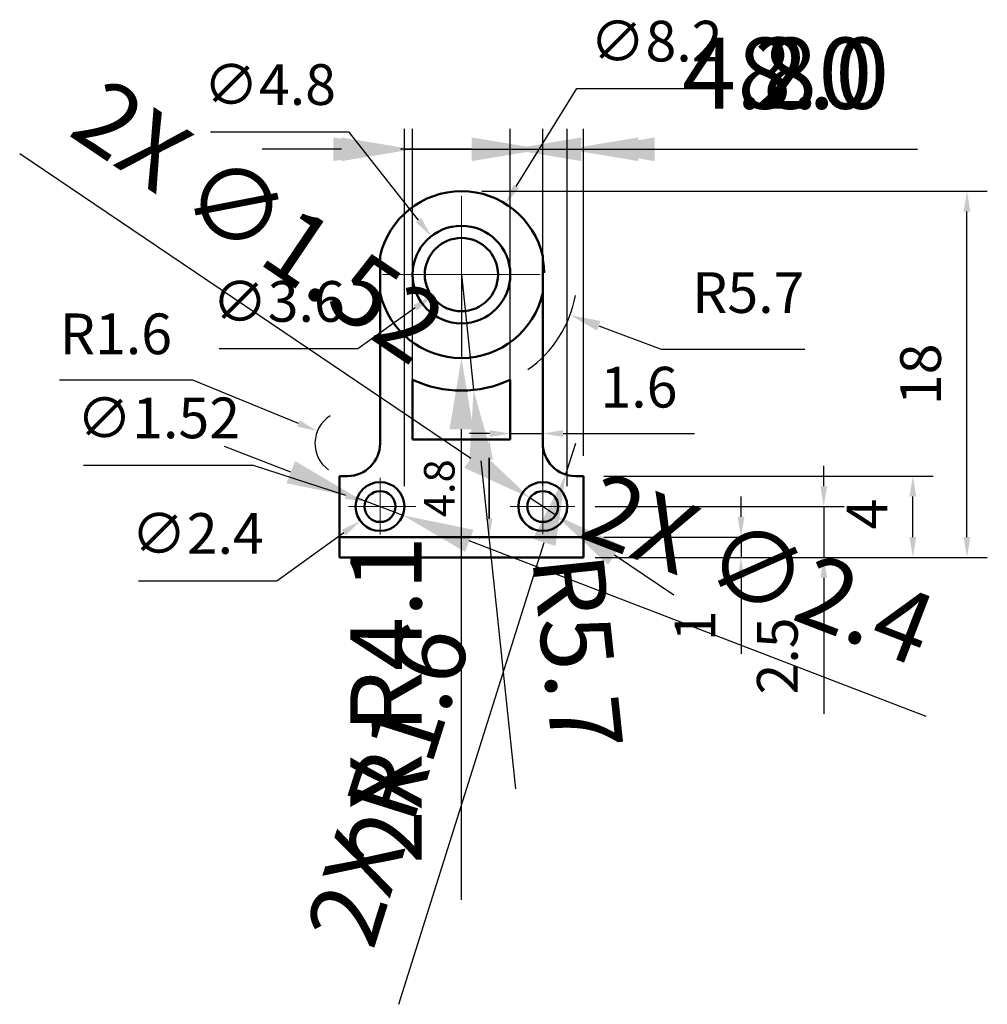
# Model space of a CAD drawing. Units: millimetres. Extents: x -15.7 to 31.8, y -22 to 26.4.
import ezdxf

# ---------------------------------------------------------------- set-up
doc = ezdxf.new("R2010")
doc.units = ezdxf.units.MM
doc.linetypes.add('CENTER', pattern=[50.8, 31.75, -6.35, 6.35, -6.35])
for name, color, linetype, lineweight in [('M-CNTR', 4, 'CENTER', 18), ('M-DIMS', 3, 'Continuous', 25), ('M-OUTL', 7, 'Continuous', 50)]:
    doc.layers.add(name, color=color, linetype=linetype, lineweight=lineweight)
doc.styles.get("Standard").update_dxf_attribs({"font": 'arial.ttf'})
doc.dimstyles.new('AM_ISO$0', dxfattribs={"dimtxt": 3.5, "dimasz": 3.5, "dimexe": 1, "dimexo": 1, "dimgap": 1.5, "dimtad": 1, "dimdsep": 46, "dimtxsty": 'Standard', "dimcen": 0, "dimclrd": 256, "dimclre": 256, "dimclrt": 2, "dimadec": 0, "dimazin": 2, "dimtp": 0.1, "dimtm": 0.1, "dimtfac": 0.71, "dimtdec": 3, "dimtmove": 0, "dimatfit": 3, "dimfxl": 1, "dimlwd": -1, "dimlwe": -1, "dimarcsym": 1})
doc.dimstyles.new('AM_ISO$3', dxfattribs={"dimtxt": 3.5, "dimasz": 3.5, "dimexe": 1, "dimexo": 1, "dimgap": 1.5, "dimtad": 1, "dimtoh": 1, "dimdsep": 46, "dimtxsty": 'Standard', "dimcen": 0, "dimclrd": 256, "dimclre": 256, "dimclrt": 2, "dimadec": 0, "dimazin": 2, "dimtp": 0.1, "dimtm": 0.1, "dimtfac": 0.71, "dimtdec": 3, "dimtofl": 0, "dimtmove": 0, "dimatfit": 0, "dimfxl": 1, "dimlwd": -1, "dimlwe": -1, "dimarcsym": 1})
doc.dimstyles.new('AM_ISO$4', dxfattribs={"dimtxt": 3.5, "dimasz": 3.5, "dimexe": 1, "dimexo": 1, "dimgap": 1.5, "dimtad": 1, "dimtoh": 1, "dimdsep": 46, "dimtxsty": 'Standard', "dimcen": 0, "dimclrd": 256, "dimclre": 256, "dimclrt": 2, "dimadec": 0, "dimazin": 2, "dimtp": 0.1, "dimtm": 0.1, "dimtfac": 0.71, "dimtdec": 3, "dimtofl": 0, "dimtmove": 0, "dimatfit": 0, "dimfxl": 1, "dimlwd": -1, "dimlwe": -1, "dimarcsym": 1})

# ---------------------------------------------------------------- blocks, each defined once
blk = doc.blocks.new('*D3')
at = {"layer": 'Defpoints', "color": 0, "transparency": 16777216}
for p in [(-1.081, 6.205), (0.4, 5.6)]:
    blk.add_point(p, dxfattribs=at)
at = {"layer": 'M-DIMS', "color": 0, "linetype": 'ByBlock', "transparency": 16777216}
for p, q in [((-7.207, 8.709), (-13.761, 8.709)), ((-2.007, 6.584), (-7.207, 8.709))]:
    blk.add_line(p, q, dxfattribs=at)
blk.add_arc((0.4, 5.6), 1.6, 121.9633, 234.1901, dxfattribs=at)
at = {"layer": 'M-DIMS', "color": 0, "transparency": 16777216}
blk.add_solid([(-1.944, 6.738), (-2.07, 6.429), (-1.081, 6.205)], dxfattribs=at)
at = {"layer": 'M-DIMS', "color": 0, "transparency": 16777216, "insert": (-10.984, 10.73), "char_height": 2, "attachment_point": 5}
blk.add_mtext('R1.6', dxfattribs=at)
blk = doc.blocks.new('*D4')
at = {"layer": 'Defpoints', "color": 0, "transparency": 16777216}
for p in [(6, 18), (30.85, 18), (12, 0)]:
    blk.add_point(p, dxfattribs=at)
at = {"layer": 'M-DIMS', "color": 0, "linetype": 'ByBlock', "transparency": 16777216}
for p, q in [((7, 18), (31.85, 18)), ((30.85, 1), (30.85, 17)), ((13, 0), (31.85, 0))]:
    blk.add_line(p, q, dxfattribs=at)
at = {"layer": 'M-DIMS', "color": 0, "transparency": 16777216}
for points in [[(30.683, 17), (31.016, 17), (30.85, 18)], [(30.683, 1), (31.016, 1), (30.85, 0)]]:
    blk.add_solid(points, dxfattribs=at)
at = {"layer": 'M-DIMS', "color": 0, "transparency": 16777216, "insert": (28.828, 9), "char_height": 2, "attachment_point": 5, "rotation": 90}
blk.add_mtext('18', dxfattribs=at)
blk = doc.blocks.new('*D5')
at = {"layer": 'Defpoints', "color": 0, "transparency": 16777216}
for p in [(12, 4), (28.191, 4), (12, 0)]:
    blk.add_point(p, dxfattribs=at)
at = {"layer": 'M-DIMS', "color": 0, "linetype": 'ByBlock', "transparency": 16777216}
for p, q in [((13, 4), (29.191, 4)), ((28.191, 1), (28.191, 3)), ((13, 0), (29.191, 0))]:
    blk.add_line(p, q, dxfattribs=at)
at = {"layer": 'M-DIMS', "color": 0, "transparency": 16777216}
for points in [[(28.024, 3), (28.357, 3), (28.191, 4)], [(28.024, 1), (28.357, 1), (28.191, 0)]]:
    blk.add_solid(points, dxfattribs=at)
at = {"layer": 'M-DIMS', "color": 0, "transparency": 16777216, "insert": (26.191, 2.127), "char_height": 2, "attachment_point": 5, "rotation": 90}
blk.add_mtext('4', dxfattribs=at)
blk = doc.blocks.new('*D6')
at = {"layer": 'Defpoints', "color": 0, "transparency": 16777216}
for p in [(11.577, 2.5), (11.577, 0), (23.809, 0)]:
    blk.add_point(p, dxfattribs=at)
at = {"layer": 'M-DIMS', "color": 0, "linetype": 'ByBlock', "transparency": 16777216}
for p, q in [((23.809, 3.5), (23.809, 4.5)), ((12.577, 2.5), (24.809, 2.5)), ((23.809, 2.5), (23.809, 0)), ((12.577, 0), (24.809, 0)), ((23.809, -1), (23.809, -7.69))]:
    blk.add_line(p, q, dxfattribs=at)
at = {"layer": 'M-DIMS', "color": 0, "transparency": 16777216}
for points in [[(23.643, 3.5), (23.976, 3.5), (23.809, 2.5)], [(23.643, -1), (23.976, -1), (23.809, 0)]]:
    blk.add_solid(points, dxfattribs=at)
at = {"layer": 'M-DIMS', "color": 0, "transparency": 16777216, "insert": (21.788, -4.845), "char_height": 2, "attachment_point": 5, "rotation": 90}
blk.add_mtext('2.5', dxfattribs=at)
blk = doc.blocks.new('*D7')
at = {"layer": 'Defpoints', "color": 0, "transparency": 16777216}
for p in [(12, 1), (19.744, 1), (12, 0)]:
    blk.add_point(p, dxfattribs=at)
at = {"layer": 'M-DIMS', "color": 0, "linetype": 'ByBlock', "transparency": 16777216}
for p, q in [((19.744, 2), (19.744, 3)), ((13, 1), (20.744, 1)), ((19.744, 1), (19.744, 0)), ((13, 0), (20.744, 0)), ((19.744, -1), (19.744, -4.737))]:
    blk.add_line(p, q, dxfattribs=at)
at = {"layer": 'M-DIMS', "color": 0, "transparency": 16777216}
for points in [[(19.577, 2), (19.911, 2), (19.744, 1)], [(19.577, -1), (19.911, -1), (19.744, 0)]]:
    blk.add_solid(points, dxfattribs=at)
at = {"layer": 'M-DIMS', "color": 0, "transparency": 16777216, "insert": (17.74, -3.368), "char_height": 2, "attachment_point": 5, "rotation": 90}
blk.add_mtext('1', dxfattribs=at)
blk = doc.blocks.new('*D8')
at = {"layer": 'Defpoints', "color": 0, "transparency": 16777216}
for p in [(10, 6.087), (8.4, 5.8), (10, 5.8)]:
    blk.add_point(p, dxfattribs=at)
at = {"layer": 'M-DIMS', "color": 0, "linetype": 'ByBlock', "transparency": 16777216}
for p, q in [((8.4, 6.8), (8.4, 7.087)), ((10, 6.8), (10, 7.087)), ((7.4, 6.087), (6.4, 6.087)), ((8.4, 6.087), (10, 6.087)), ((11, 6.087), (17.452, 6.087))]:
    blk.add_line(p, q, dxfattribs=at)
at = {"layer": 'M-DIMS', "color": 0, "transparency": 16777216}
for points in [[(7.4, 6.254), (7.4, 5.92), (8.4, 6.087)], [(11, 6.254), (11, 5.92), (10, 6.087)]]:
    blk.add_solid(points, dxfattribs=at)
at = {"layer": 'M-DIMS', "color": 0, "transparency": 16777216, "insert": (14.726, 8.108), "char_height": 2, "attachment_point": 5}
blk.add_mtext('1.6', dxfattribs=at)
blk = doc.blocks.new('*D9')
at = {"layer": 'Defpoints', "color": 0, "transparency": 16777216}
for p in [(2.973, 3.203), (1.027, 1.797)]:
    blk.add_point(p, dxfattribs=at)
at = {"layer": 'M-DIMS', "color": 0, "linetype": 'ByBlock', "transparency": 16777216}
for p, q in [((0.217, 1.212), (-3.067, -1.161)), ((-3.067, -1.161), (-9.876, -1.161))]:
    blk.add_line(p, q, dxfattribs=at)
at = {"layer": 'M-DIMS', "color": 0, "transparency": 16777216}
blk.add_solid([(0.119, 1.347), (0.314, 1.077), (1.027, 1.797)], dxfattribs=at)
at = {"layer": 'M-DIMS', "color": 0, "transparency": 16777216, "insert": (-6.972, 0.916), "char_height": 2, "attachment_point": 5}
blk.add_mtext('∅2.4', dxfattribs=at)
blk = doc.blocks.new('*D10')
at = {"layer": 'Defpoints', "color": 0, "transparency": 16777216}
for p in [(1.277, 2.735), (2.723, 2.265)]:
    blk.add_point(p, dxfattribs=at)
at = {"layer": 'M-DIMS', "color": 0, "linetype": 'ByBlock', "transparency": 16777216}
for p, q in [((-4.223, 4.521), (-12.573, 4.521)), ((0.326, 3.044), (-4.223, 4.521))]:
    blk.add_line(p, q, dxfattribs=at)
at = {"layer": 'M-DIMS', "color": 0, "transparency": 16777216}
blk.add_solid([(0.378, 3.202), (0.275, 2.885), (1.277, 2.735)], dxfattribs=at)
at = {"layer": 'M-DIMS', "color": 0, "transparency": 16777216, "insert": (-8.898, 6.598), "char_height": 2, "attachment_point": 5}
blk.add_mtext('∅1.52', dxfattribs=at)
blk = doc.blocks.new('*D11')
at = {"layer": 'Defpoints', "color": 0, "transparency": 16777216}
for p in [(7.462, 14.95), (4.538, 12.85)]:
    blk.add_point(p, dxfattribs=at)
at = {"layer": 'M-DIMS', "color": 0, "linetype": 'ByBlock', "transparency": 16777216}
for p, q in [((3.726, 12.266), (0.914, 10.246)), ((0.914, 10.246), (-5.902, 10.246))]:
    blk.add_line(p, q, dxfattribs=at)
at = {"layer": 'M-DIMS', "color": 0, "transparency": 16777216}
blk.add_solid([(3.629, 12.401), (3.823, 12.131), (4.538, 12.85)], dxfattribs=at)
at = {"layer": 'M-DIMS', "color": 0, "transparency": 16777216, "insert": (-2.994, 12.323), "char_height": 2, "attachment_point": 5}
blk.add_mtext('∅3.6', dxfattribs=at)
blk = doc.blocks.new('*D12')
at = {"layer": 'Defpoints', "color": 0, "transparency": 16777216}
for p in [(4.516, 15.786), (7.484, 12.014)]:
    blk.add_point(p, dxfattribs=at)
at = {"layer": 'M-DIMS', "color": 0, "linetype": 'ByBlock', "transparency": 16777216}
for p, q in [((0.487, 20.904), (-6.335, 20.904)), ((3.897, 16.572), (0.487, 20.904))]:
    blk.add_line(p, q, dxfattribs=at)
at = {"layer": 'M-DIMS', "color": 0, "transparency": 16777216}
blk.add_solid([(4.028, 16.675), (3.766, 16.469), (4.516, 15.786)], dxfattribs=at)
at = {"layer": 'M-DIMS', "color": 0, "transparency": 16777216, "insert": (-3.424, 22.982), "char_height": 2, "attachment_point": 5}
blk.add_mtext('∅4.8', dxfattribs=at)
blk = doc.blocks.new('*D13')
at = {"layer": 'Defpoints', "color": 0, "transparency": 16777216}
for p in [(8.164, 17.383), (3.836, 10.417)]:
    blk.add_point(p, dxfattribs=at)
at = {"layer": 'M-DIMS', "color": 0, "linetype": 'ByBlock', "transparency": 16777216}
for p, q in [((8.691, 18.232), (11.678, 23.041)), ((11.678, 23.041), (18.475, 23.041))]:
    blk.add_line(p, q, dxfattribs=at)
blk.add_arc((6, 13.9), 4.1, 1.2942, 72.1254, dxfattribs=at)
at = {"layer": 'M-DIMS', "color": 0, "transparency": 16777216}
blk.add_solid([(8.55, 18.32), (8.833, 18.144), (8.164, 17.383)], dxfattribs=at)
at = {"layer": 'M-DIMS', "color": 0, "transparency": 16777216, "insert": (15.577, 25.118), "char_height": 2, "attachment_point": 5}
blk.add_mtext('∅8.2', dxfattribs=at)
blk = doc.blocks.new('*D14')
at = {"layer": 'Defpoints', "color": 0, "transparency": 16777216}
for p in [(6, 5.8), (7.371, 5.8), (6, 1)]:
    blk.add_point(p, dxfattribs=at)
at = {"layer": 'M-DIMS', "color": 0, "linetype": 'ByBlock', "transparency": 16777216}
for p, q in [((7, 5.8), (8.371, 5.8)), ((7, 1), (8.371, 1))]:
    blk.add_line(p, q, dxfattribs=at)
at = {"layer": 'M-DIMS', "color": 0, "linetype": 'ByBlock', "lineweight": 35, "transparency": 16777216}
blk.add_line((7.371, 1.9), (7.371, 4.9), dxfattribs=at)
at = {"layer": 'M-DIMS', "color": 0, "transparency": 16777216}
for points in [[(7.221, 4.9), (7.521, 4.9), (7.371, 5.8)], [(7.221, 1.9), (7.521, 1.9), (7.371, 1)]]:
    blk.add_solid(points, dxfattribs=at)
at = {"layer": 'M-DIMS', "color": 0, "transparency": 16777216, "insert": (5.105, 3.4), "char_height": 1.5, "attachment_point": 5, "rotation": 90}
blk.add_mtext('4.8', dxfattribs=at)
blk = doc.blocks.new('*D15')
at = {"layer": 'Defpoints', "color": 0, "transparency": 16777216}
for p in [(6, 13.9), (11.341, 11.91)]:
    blk.add_point(p, dxfattribs=at)
at = {"layer": 'M-DIMS', "color": 0, "linetype": 'ByBlock', "transparency": 16777216}
for p, q in [((12.747, 11.386), (15.822, 10.241)), ((15.822, 10.241), (22.878, 10.241))]:
    blk.add_line(p, q, dxfattribs=at)
blk.add_arc((6, 13.9), 5.7, 304.953, 349.6183, dxfattribs=at)
at = {"layer": 'M-DIMS', "color": 0, "transparency": 16777216}
blk.add_solid([(12.834, 11.621), (12.66, 11.152), (11.341, 11.91)], dxfattribs=at)
at = {"layer": 'M-DIMS', "color": 0, "transparency": 16777216, "insert": (20.1, 12.758), "char_height": 2, "attachment_point": 5}
blk.add_mtext('R5.7', dxfattribs=at)
blk = doc.blocks.new('MOUNT-HOLE-D1_52-D2_40')
for radius in [1.2, 0.76]:
    blk.add_circle((0, 0), radius)
blk = doc.blocks.new('*D17')
at = {"layer": 'Defpoints', "color": 0, "transparency": 16777216}
for p in [(12, 20.06), (12, 4), (10, 2.5)]:
    blk.add_point(p, dxfattribs=at)
at = {"layer": 'M-DIMS', "linetype": 'ByBlock', "transparency": 16777216}
for p, q in [((10, 3.5), (10, 21.06)), ((12, 5), (12, 21.06)), ((6.5, 20.06), (3, 20.06)), ((10, 20.06), (12, 20.06)), ((15.5, 20.06), (28.42, 20.06))]:
    blk.add_line(p, q, dxfattribs=at)
at = {"layer": 'M-DIMS', "transparency": 16777216}
for points in [[(6.5, 20.643), (6.5, 19.477), (10, 20.06)], [(15.5, 20.643), (15.5, 19.477), (12, 20.06)]]:
    blk.add_solid(points, dxfattribs=at)
at = {"layer": 'M-DIMS', "color": 2, "transparency": 16777216, "insert": (23.71, 23.347), "char_height": 3.5, "attachment_point": 5}
blk.add_mtext('2.0', dxfattribs=at)
blk = doc.blocks.new('*D18')
at = {"layer": 'Defpoints', "color": 0, "transparency": 16777216}
for p in [(11.2, 20.06), (3.2, 2.5), (11.2, 2.5)]:
    blk.add_point(p, dxfattribs=at)
at = {"layer": 'M-DIMS', "linetype": 'ByBlock', "transparency": 16777216}
for p, q in [((3.2, 3.5), (3.2, 21.06)), ((11.2, 3.5), (11.2, 21.06)), ((-0.3, 20.06), (-3.8, 20.06)), ((3.2, 20.06), (11.2, 20.06)), ((14.7, 20.06), (27.565, 20.06))]:
    blk.add_line(p, q, dxfattribs=at)
at = {"layer": 'M-DIMS', "transparency": 16777216}
for points in [[(-0.3, 20.643), (-0.3, 19.477), (3.2, 20.06)], [(14.7, 20.643), (14.7, 19.477), (11.2, 20.06)]]:
    blk.add_solid(points, dxfattribs=at)
at = {"layer": 'M-DIMS', "color": 2, "transparency": 16777216, "insert": (22.882, 23.347), "char_height": 3.5, "attachment_point": 5}
blk.add_mtext('8.0', dxfattribs=at)
blk = doc.blocks.new('*D19')
at = {"layer": 'Defpoints', "color": 0, "transparency": 16777216}
for p in [(8.4, 20.06), (3.6, 5.8), (8.4, 5.8)]:
    blk.add_point(p, dxfattribs=at)
at = {"layer": 'M-DIMS', "linetype": 'ByBlock', "transparency": 16777216}
for p, q in [((3.6, 6.8), (3.6, 21.06)), ((8.4, 6.8), (8.4, 21.06)), ((0.1, 20.06), (-3.4, 20.06)), ((3.6, 20.06), (8.4, 20.06)), ((11.9, 20.06), (24.92, 20.06))]:
    blk.add_line(p, q, dxfattribs=at)
at = {"layer": 'M-DIMS', "transparency": 16777216}
for points in [[(0.1, 20.643), (0.1, 19.477), (3.6, 20.06)], [(11.9, 20.643), (11.9, 19.477), (8.4, 20.06)]]:
    blk.add_solid(points, dxfattribs=at)
at = {"layer": 'M-DIMS', "color": 2, "transparency": 16777216, "insert": (20.16, 23.347), "char_height": 3.5, "attachment_point": 5}
blk.add_mtext('4.8', dxfattribs=at)
blk = doc.blocks.new('*D20')
at = {"layer": 'Defpoints', "color": 0, "transparency": 16777216}
for p in [(6, 13.9), (6, 9.8)]:
    blk.add_point(p, dxfattribs=at)
at = {"layer": 'M-DIMS', "linetype": 'ByBlock', "transparency": 16777216}
for p, q in [((6, 13.9), (6, 9.8)), ((6, -16.826), (6, 6.3))]:
    blk.add_line(p, q, dxfattribs=at)
at = {"layer": 'M-DIMS', "transparency": 16777216}
blk.add_solid([(5.417, 6.3), (6.583, 6.3), (6, 9.8)], dxfattribs=at)
at = {"layer": 'M-DIMS', "color": 2, "transparency": 16777216, "insert": (2.742, -7.013), "char_height": 3.5, "attachment_point": 5, "rotation": 90}
blk.add_mtext('2X R4.1', dxfattribs=at)
blk = doc.blocks.new('*D21')
at = {"layer": 'Defpoints', "color": 0, "transparency": 16777216}
for p in [(6, 13.9), (6.6, 8.232)]:
    blk.add_point(p, dxfattribs=at)
at = {"layer": 'M-DIMS', "linetype": 'ByBlock', "transparency": 16777216}
for p, q in [((6, 13.9), (6.6, 8.232)), ((8.676, -11.38), (6.968, 4.751))]:
    blk.add_line(p, q, dxfattribs=at)
at = {"layer": 'M-DIMS', "transparency": 16777216}
blk.add_solid([(7.549, 4.813), (6.388, 4.69), (6.6, 8.232)], dxfattribs=at)
at = {"layer": 'M-DIMS', "color": 2, "transparency": 16777216, "insert": (11.268, -4.71), "char_height": 3.5, "attachment_point": 5, "rotation": 276.0427}
blk.add_mtext('R5.7', dxfattribs=at)
blk = doc.blocks.new('*D22')
at = {"layer": 'Defpoints', "color": 0, "transparency": 16777216}
for p in [(11.6, 5.6), (11.12, 4.074)]:
    blk.add_point(p, dxfattribs=at)
at = {"layer": 'M-DIMS', "linetype": 'ByBlock', "transparency": 16777216}
for p, q in [((11.6, 5.6), (11.12, 4.074)), ((2.929, -21.968), (10.07, 0.735))]:
    blk.add_line(p, q, dxfattribs=at)
at = {"layer": 'M-DIMS', "transparency": 16777216}
blk.add_solid([(9.513, 0.91), (10.626, 0.56), (11.12, 4.074)], dxfattribs=at)
at = {"layer": 'M-DIMS', "color": 2, "transparency": 16777216, "insert": (2.839, -11.299), "char_height": 3.5, "attachment_point": 5, "rotation": 72.5391}
blk.add_mtext('2X R1.6', dxfattribs=at)
blk = doc.blocks.new('*D23')
at = {"layer": 'Defpoints', "color": 0, "transparency": 16777216}
for p in [(0.88, 2.931), (3.12, 2.069)]:
    blk.add_point(p, dxfattribs=at)
at = {"layer": 'M-DIMS', "linetype": 'ByBlock', "transparency": 16777216}
for p, q in [((-2.386, 4.188), (-5.653, 5.445)), ((0.88, 2.931), (3.12, 2.069)), ((28.841, -7.829), (6.386, 0.812))]:
    blk.add_line(p, q, dxfattribs=at)
at = {"layer": 'M-DIMS', "transparency": 16777216}
for points in [[(-2.177, 4.732), (-2.596, 3.644), (0.88, 2.931)], [(6.596, 1.356), (6.177, 0.268), (3.12, 2.069)]]:
    blk.add_solid(points, dxfattribs=at)
at = {"layer": 'M-DIMS', "color": 2, "transparency": 16777216, "insert": (20.463, -0.978), "char_height": 3.5, "attachment_point": 5, "rotation": 338.9522}
blk.add_mtext('2X ∅2.4', dxfattribs=at)
blk = doc.blocks.new('*D24')
at = {"layer": 'Defpoints', "color": 0, "transparency": 16777216}
for p in [(9.37, 2.925), (10.63, 2.075)]:
    blk.add_point(p, dxfattribs=at)
at = {"layer": 'M-DIMS', "linetype": 'ByBlock', "transparency": 16777216}
for p, q in [((-15.714, 19.846), (6.468, 4.882)), ((10.63, 2.075), (9.37, 2.925)), ((13.532, 0.118), (16.433, -1.84))]:
    blk.add_line(p, q, dxfattribs=at)
at = {"layer": 'M-DIMS', "transparency": 16777216}
for points in [[(6.795, 5.366), (6.142, 4.399), (9.37, 2.925)], [(13.858, 0.601), (13.205, -0.366), (10.63, 2.075)]]:
    blk.add_solid(points, dxfattribs=at)
at = {"layer": 'M-DIMS', "color": 2, "transparency": 16777216, "insert": (-4.18, 16.149), "char_height": 3.5, "attachment_point": 5, "rotation": 325.9963}
blk.add_mtext('2X ∅1.52', dxfattribs=at)

msp = doc.modelspace()

# ---------------------------------------------------------------- linework, layer by layer
at = {"layer": 'M-CNTR'}
for p, q in [((6, 10.023), (6, 17.777)), ((2.123, 13.9), (9.877, 13.9)), ((2, 1.129), (2, 3.915)), ((10, 1.144), (10, 4.132)), ((0.452, 2.5), (3.756, 2.5)), ((8.396, 2.5), (11.577, 2.5))]:
    msp.add_line(p, q, dxfattribs=at)
at = {"layer": 'M-OUTL'}
for p, q in [((2, 5.6), (2, 14.8)), ((10, 5.6), (10, 14.8)), ((3.6, 5.8), (3.6, 8.73)), ((8.4, 5.8), (8.4, 8.73)), ((3.6, 5.8), (8.4, 5.8)), ((0, 0), (0, 4)), ((0, 4), (0.4, 4)), ((12, 4), (11.6, 4)), ((12, 0), (12, 4)), ((0, 1), (12, 1)), ((0, 0), (12, 0))]:
    msp.add_line(p, q, dxfattribs=at)
for radius in [2.4, 1.8]:
    msp.add_circle((6, 13.9), radius, dxfattribs=at)
for centre, radius, start, end in [((6, 13.9), 4.1, 12.6804, 167.3196), ((6, 13.9), 4.1, 192.6804, 347.3196), ((6, 13.9), 5.7, 245.0989, 294.9011), ((0.4, 5.6), 1.6, 270, 0), ((11.6, 5.6), 1.6, 180, 270)]:
    msp.add_arc(centre, radius, start, end, dxfattribs=at)

# ---------------------------------------------------------------- block references
for p in [(2, 2.5), (10, 2.5)]:
    msp.add_blockref('MOUNT-HOLE-D1_52-D2_40', p, dxfattribs=at)

# ---------------------------------------------------------------- dimensions: what is measured, and where the dimension line sits
at = {"layer": 'M-DIMS'}
for p1, p2, picture, middle in [((3.836, 10.417), (8.164, 17.383), '*D13', (15.577, 23.041)), ((7.484, 12.014), (4.516, 15.786), '*D12', (-3.424, 20.904)), ((7.462, 14.95), (4.538, 12.85), '*D11', (-2.994, 10.246)), ((2.723, 2.265), (1.277, 2.735), '*D10', (-8.898, 4.521)), ((2.973, 3.203), (1.027, 1.797), '*D9', (-6.972, -1.161))]:
    dim = msp.add_diameter_dim_2p(p1=p1, p2=p2, dimstyle='AM_ISO$3', override={"dimtxt": 2, "dimasz": 1, "dimgap": 1, "dimclrd": 0, "dimclre": 0, "dimclrt": 0}, dxfattribs=at)
    dim.commit()
    dim.dimension.update_dxf_attribs({"geometry": picture, "text_midpoint": middle, "dimtype": 163})
for base, p1, p2, picture, middle in [((11.2, 20.06), (3.2, 2.5), (11.2, 2.5), '*D18', (22.882, 23.347)), ((8.4, 20.06), (3.6, 5.8), (8.4, 5.8), '*D19', (20.16, 23.347)), ((12, 20.06), (10, 2.5), (12, 4), '*D17', (23.71, 23.347))]:
    dim = msp.add_linear_dim(base=base, p1=p1, p2=p2, dimstyle='AM_ISO$0', override={"dimdec": 1, "dimlfac": 1, "dimrnd": 0, "dimzin": 0, "dimdsep": 46, "dimlunit": 2}, dxfattribs=at)
    dim.commit()
    dim.dimension.update_dxf_attribs({"geometry": picture, "text_midpoint": middle})
for p1, p2, override, picture, middle in [((10.63, 2.075), (9.37, 2.925), {"dimdec": 2, "dimlfac": 1, "dimrnd": 0, "dimzin": 0, "dimdsep": 46, "dimlunit": 2}, '*D24', (-6.073, 13.343)), ((0.88, 2.931), (3.12, 2.069), {"dimdec": 1, "dimlfac": 1, "dimrnd": 0, "dimzin": 0, "dimdsep": 46, "dimlunit": 2}, '*D23', (19.247, -4.137))]:
    dim = msp.add_diameter_dim_2p(p1=p1, p2=p2, text='2X <>', dimstyle='AM_ISO$0', override=override, dxfattribs=at)
    dim.commit()
    dim.dimension.update_dxf_attribs({"geometry": picture, "text_midpoint": middle, "dimtype": 163})
for base, p1, p2, override, picture, middle in [((30.85, 18), (12, 0), (6, 18), {"dimtxt": 2, "dimasz": 1, "dimgap": 1, "dimclrd": 0, "dimclre": 0, "dimclrt": 0}, '*D4', (30.85, 9)), ((7.371, 5.8), (6, 1), (6, 5.8), {"dimtxt": 1.5, "dimasz": 0.9, "dimclrd": 0, "dimclre": 0, "dimclrt": 0, "dimlwd": 35}, '*D14', (7.371, 3.4)), ((23.809, 0), (11.577, 2.5), (11.577, 0), {"dimtxt": 2, "dimasz": 1, "dimgap": 1, "dimclrd": 0, "dimclre": 0, "dimclrt": 0}, '*D6', (23.809, -4.845)), ((28.191, 4), (12, 0), (12, 4), {"dimtxt": 2, "dimasz": 1, "dimgap": 1, "dimclrd": 0, "dimclre": 0, "dimclrt": 0}, '*D5', (28.191, 2.127)), ((19.744, 1), (12, 0), (12, 1), {"dimtxt": 2, "dimasz": 1, "dimgap": 1, "dimclrd": 0, "dimclre": 0, "dimclrt": 0}, '*D7', (19.744, -3.368))]:
    dim = msp.add_linear_dim(base=base, p1=p1, p2=p2, angle=90, dimstyle='AM_ISO$0', override=override, dxfattribs=at)
    dim.commit()
    dim.dimension.update_dxf_attribs({"geometry": picture, "text_midpoint": middle, "dimtype": 160})
for center, mpoint, override, picture, middle in [((6, 13.9), (11.341, 11.91), {"dimtxt": 2, "dimasz": 1.5, "dimclrd": 0, "dimclre": 0, "dimclrt": 0}, '*D15', (20.1, 10.241)), ((0.4, 5.6), (-1.081, 6.205), {"dimtxt": 2, "dimasz": 1, "dimgap": 1, "dimclrd": 0, "dimclre": 0, "dimclrt": 0}, '*D3', (-10.984, 8.709))]:
    dim = msp.add_radius_dim(center=center, mpoint=mpoint, dimstyle='AM_ISO$4', override=override, dxfattribs=at)
    dim.commit()
    dim.dimension.update_dxf_attribs({"geometry": picture, "text_midpoint": middle, "dimtype": 164})
for center, mpoint, picture, middle in [((6, 13.9), (6, 9.8), '*D20', (2.742, -7.013)), ((11.6, 5.6), (11.12, 4.074), '*D22', (2.839, -11.299))]:
    dim = msp.add_radius_dim(center=center, mpoint=mpoint, text='2X <>', dimstyle='AM_ISO$0', override={"dimdec": 1, "dimlfac": 1, "dimrnd": 0, "dimzin": 0, "dimdsep": 46, "dimlunit": 2}, dxfattribs=at)
    dim.commit()
    dim.dimension.update_dxf_attribs({"geometry": picture, "text_midpoint": middle})
dim = msp.add_radius_dim(center=(6, 13.9), mpoint=(6.6, 8.232), dimstyle='AM_ISO$0', override={"dimdec": 1, "dimlfac": 1, "dimrnd": 0, "dimzin": 0, "dimdsep": 46, "dimlunit": 2}, dxfattribs=at)
dim.commit()
dim.dimension.update_dxf_attribs({"geometry": '*D21', "text_midpoint": (11.268, -4.71)})
dim = msp.add_linear_dim(base=(10, 6.087), p1=(8.4, 5.8), p2=(10, 5.8), dimstyle='AM_ISO$0', override={"dimtxt": 2, "dimasz": 1, "dimgap": 1, "dimclrd": 0, "dimclre": 0, "dimclrt": 0}, dxfattribs=at)
dim.commit()
dim.dimension.update_dxf_attribs({"geometry": '*D8', "text_midpoint": (14.726, 6.087), "dimtype": 160})

doc.saveas('drawing.dxf')
